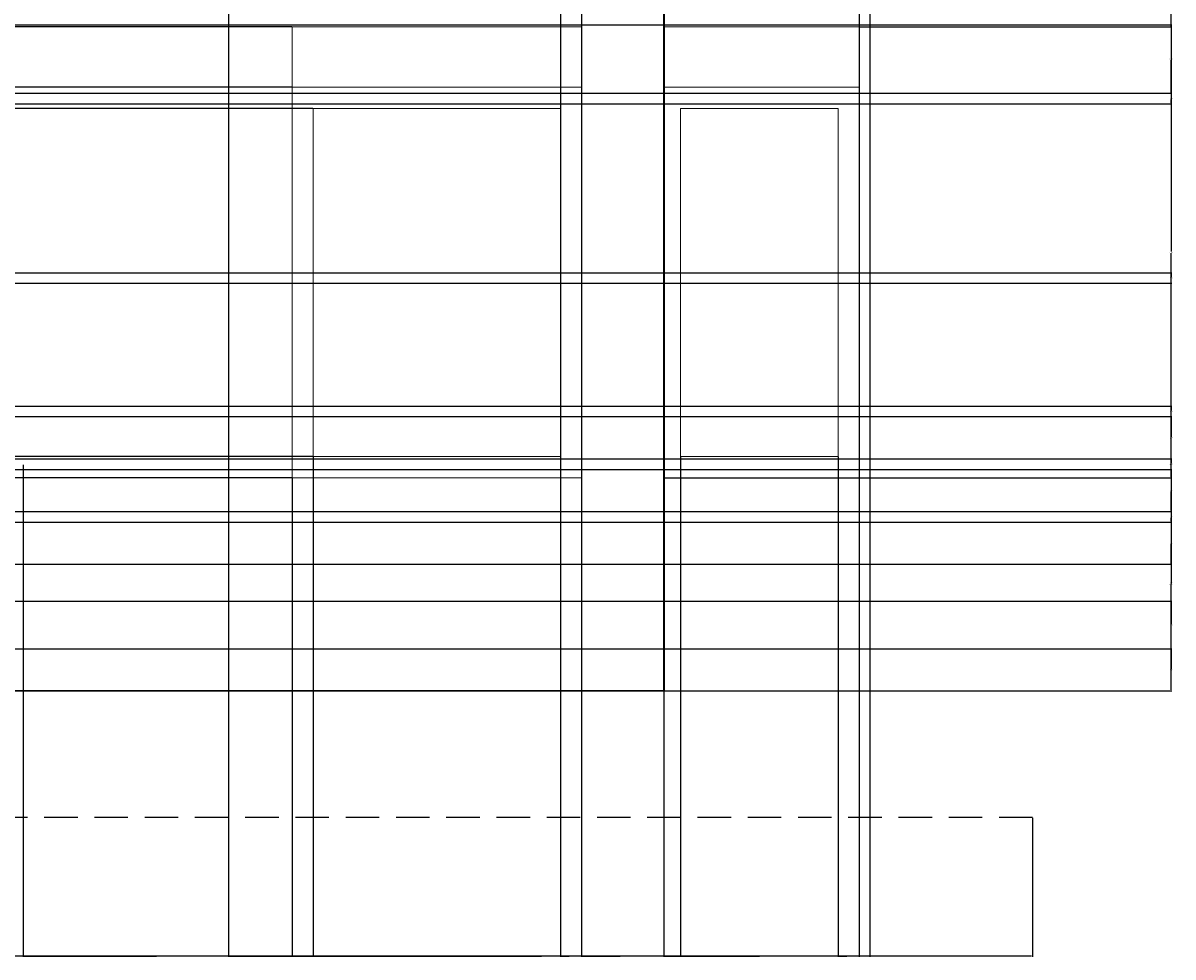
# Model space of a CAD drawing. Units: inches. Extents: x 1817 to 2378, y 1915 to 2370.
# Tile 6 of 8: x 2160 to 2378, y 1915 to 2092. Entities that reach past the tile are written whole.
import ezdxf

# ---------------------------------------------------------------- set-up
doc = ezdxf.new("R2010")
doc.units = ezdxf.units.IN
doc.linetypes.add('DASHED', pattern=[19.05, 12.7, -6.35])
doc.linetypes.add('DASHED2', pattern=[9.525, 6.35, -3.175])
for name, color, linetype, lineweight in [('A-ANNO-DIMS', 2, 'Continuous', 18), ('A-ELEV', 7, 'Continuous', 35), ('A-ELEV-HIDN', 8, 'DASHED', 18), ('A-GLAZ', 4, 'Continuous', 18), ('C-TOPO', 8, 'DASHED2', 25)]:
    doc.layers.add(name, color=color, linetype=linetype, lineweight=lineweight)
doc.styles.get("Standard").update_dxf_attribs({"font": 'arial.ttf'})
doc.dimstyles.get("Standard").update_dxf_attribs({"dimtxt": 0.18, "dimasz": 0.18, "dimexe": 0.18, "dimexo": 0.0625, "dimgap": 0.09, "dimtad": 0, "dimtih": 1, "dimtoh": 1, "dimdec": 4, "dimzin": 0, "dimdsep": 46, "dimtxsty": 'Standard', "dimcen": 0.09, "dimadec": 0, "dimazin": 0, "dimtfac": 1, "dimtdec": 4, "dimtofl": 0, "dimtmove": 0, "dimatfit": 3, "dimfxl": 1, "dimtolj": 1, "dimtzin": 0, "dimarcsym": 0})

# ---------------------------------------------------------------- blocks, each defined once
blk = doc.blocks.new('*D19')
at = {"layer": 'A-ANNO-DIMS', "color": 0, "lineweight": -2, "transparency": 16777216}
for p, q in [((2159.62, 2008.38), (2159.62, 1915.08)), ((2210.62, 2005.87), (2210.62, 1915.08)), ((2159.8, 1915.26), (2184.92, 1915.26)), ((2210.44, 1915.26), (2185.32, 1915.26))]:
    blk.add_line(p, q, dxfattribs=at)
at = {"layer": 'A-ANNO-DIMS', "color": 0, "transparency": 16777216}
for points in [[(2159.8, 1915.29), (2159.8, 1915.23), (2159.62, 1915.26)], [(2210.44, 1915.29), (2210.44, 1915.23), (2210.62, 1915.26)]]:
    blk.add_solid(points, dxfattribs=at)
at = {"layer": 'Defpoints', "color": 0, "transparency": 16777216}
for p in [(2159.62, 2008.45), (2210.62, 2005.93), (2210.62, 1915.26)]:
    blk.add_point(p, dxfattribs=at)
at = {"layer": 'A-ANNO-DIMS', "color": 0, "transparency": 16777216, "insert": (2185.12, 1915.26), "char_height": 0.18, "attachment_point": 5}
blk.add_mtext('\\A1;51', dxfattribs=at)
blk = doc.blocks.new('*D20')
at = {"layer": 'A-ANNO-DIMS', "color": 0, "lineweight": -2, "transparency": 16777216}
for p, q in [((2210.62, 2005.87), (2210.62, 1915.08)), ((2265.49, 2005.87), (2265.49, 1915.08)), ((2210.8, 1915.26), (2237.66, 1915.26)), ((2265.31, 1915.26), (2238.45, 1915.26))]:
    blk.add_line(p, q, dxfattribs=at)
at = {"layer": 'A-ANNO-DIMS', "color": 0, "transparency": 16777216}
for points in [[(2210.8, 1915.29), (2210.8, 1915.23), (2210.62, 1915.26)], [(2265.31, 1915.29), (2265.31, 1915.23), (2265.49, 1915.26)]]:
    blk.add_solid(points, dxfattribs=at)
at = {"layer": 'Defpoints', "color": 0, "transparency": 16777216}
for p in [(2210.62, 2005.93), (2265.49, 2005.93), (2265.49, 1915.26)]:
    blk.add_point(p, dxfattribs=at)
at = {"layer": 'A-ANNO-DIMS', "color": 0, "transparency": 16777216, "insert": (2238.05, 1915.26), "char_height": 0.18, "attachment_point": 5}
blk.add_mtext('\\A1;54.87', dxfattribs=at)
blk = doc.blocks.new('*D21')
at = {"layer": 'A-ANNO-DIMS', "color": 0, "lineweight": -2, "transparency": 16777216}
for p, q in [((2265.49, 2005.87), (2265.49, 1915.08)), ((2281.08, 2005.87), (2281.08, 1915.08)), ((2265.67, 1915.26), (2272.83, 1915.26)), ((2280.9, 1915.26), (2273.74, 1915.26))]:
    blk.add_line(p, q, dxfattribs=at)
at = {"layer": 'A-ANNO-DIMS', "color": 0, "transparency": 16777216}
for points in [[(2265.67, 1915.29), (2265.67, 1915.23), (2265.49, 1915.26)], [(2280.9, 1915.29), (2280.9, 1915.23), (2281.08, 1915.26)]]:
    blk.add_solid(points, dxfattribs=at)
at = {"layer": 'Defpoints', "color": 0, "transparency": 16777216}
for p in [(2265.49, 2005.93), (2281.08, 2005.93), (2281.08, 1915.26)]:
    blk.add_point(p, dxfattribs=at)
at = {"layer": 'A-ANNO-DIMS', "color": 0, "transparency": 16777216, "insert": (2273.29, 1915.26), "char_height": 0.18, "attachment_point": 5}
blk.add_mtext('\\A1;15.596', dxfattribs=at)
blk = doc.blocks.new('*D22')
at = {"layer": 'A-ANNO-DIMS', "color": 0, "lineweight": -2, "transparency": 16777216}
for p, q in [((2281.08, 2005.87), (2281.08, 1915.08)), ((2318.11, 2005.87), (2318.11, 1915.08)), ((2281.26, 1915.26), (2299.2, 1915.26)), ((2317.93, 1915.26), (2299.99, 1915.26))]:
    blk.add_line(p, q, dxfattribs=at)
at = {"layer": 'A-ANNO-DIMS', "color": 0, "transparency": 16777216}
for points in [[(2281.26, 1915.29), (2281.26, 1915.23), (2281.08, 1915.26)], [(2317.93, 1915.29), (2317.93, 1915.23), (2318.11, 1915.26)]]:
    blk.add_solid(points, dxfattribs=at)
at = {"layer": 'Defpoints', "color": 0, "transparency": 16777216}
for p in [(2281.08, 2005.93), (2318.11, 2005.93), (2318.11, 1915.26)]:
    blk.add_point(p, dxfattribs=at)
at = {"layer": 'A-ANNO-DIMS', "color": 0, "transparency": 16777216, "insert": (2299.6, 1915.26), "char_height": 0.18, "attachment_point": 5}
blk.add_mtext('\\A1;37.02', dxfattribs=at)
blk = doc.blocks.new('*D23')
at = {"layer": 'A-ANNO-DIMS', "color": 0, "lineweight": -2, "transparency": 16777216}
for p, q in [((2320.11, 2156.45), (2320.11, 1915.08)), ((1867.08, 1965.45), (1867.08, 1915.08)), ((1867.26, 1915.26), (2093.3, 1915.26)), ((2319.93, 1915.26), (2093.89, 1915.26))]:
    blk.add_line(p, q, dxfattribs=at)
at = {"layer": 'A-ANNO-DIMS', "color": 0, "transparency": 16777216}
for points in [[(1867.26, 1915.29), (1867.26, 1915.23), (1867.08, 1915.26)], [(2319.93, 1915.29), (2319.93, 1915.23), (2320.11, 1915.26)]]:
    blk.add_solid(points, dxfattribs=at)
at = {"layer": 'Defpoints', "color": 0, "transparency": 16777216}
for p in [(2320.11, 2156.51), (1867.08, 1965.51), (2320.11, 1915.26)]:
    blk.add_point(p, dxfattribs=at)
at = {"layer": 'A-ANNO-DIMS', "color": 0, "transparency": 16777216, "insert": (2093.6, 1915.26), "char_height": 0.18, "attachment_point": 5}
blk.add_mtext('\\A1;453', dxfattribs=at)
blk = doc.blocks.new('*D24')
at = {"layer": 'A-ANNO-DIMS', "color": 0, "lineweight": -2, "transparency": 16777216}
for p, q in [((2198.59, 2103.51), (2198.59, 1915.08)), ((2318.11, 2103.51), (2318.11, 1915.08)), ((2198.77, 1915.26), (2257.89, 1915.26)), ((2317.93, 1915.26), (2258.8, 1915.26))]:
    blk.add_line(p, q, dxfattribs=at)
at = {"layer": 'A-ANNO-DIMS', "color": 0, "transparency": 16777216}
for points in [[(2198.77, 1915.29), (2198.77, 1915.23), (2198.59, 1915.26)], [(2317.93, 1915.29), (2317.93, 1915.23), (2318.11, 1915.26)]]:
    blk.add_solid(points, dxfattribs=at)
at = {"layer": 'Defpoints', "color": 0, "transparency": 16777216}
for p in [(2198.59, 2103.57), (2318.11, 2103.57), (2318.11, 1915.26)]:
    blk.add_point(p, dxfattribs=at)
at = {"layer": 'A-ANNO-DIMS', "color": 0, "transparency": 16777216, "insert": (2258.35, 1915.26), "char_height": 0.18, "attachment_point": 5}
blk.add_mtext('\\A1;119.52', dxfattribs=at)
blk = doc.blocks.new('*D69')
at = {"layer": 'A-ANNO-DIMS', "color": 0, "lineweight": -2, "transparency": 16777216}
for p, q in [((2281.15, 2005.93), (2377.4, 2005.93)), ((2377.22, 2005.75), (2377.22, 1985.9)), ((2377.22, 1965.69), (2377.22, 1985.54)), ((2281.15, 1965.51), (2377.4, 1965.51))]:
    blk.add_line(p, q, dxfattribs=at)
at = {"layer": 'A-ANNO-DIMS', "color": 0, "transparency": 16777216}
for points in [[(2377.19, 2005.75), (2377.25, 2005.75), (2377.22, 2005.93)], [(2377.19, 1965.69), (2377.25, 1965.69), (2377.22, 1965.51)]]:
    blk.add_solid(points, dxfattribs=at)
at = {"layer": 'Defpoints', "color": 0, "transparency": 16777216}
for p in [(2281.08, 2005.93), (2377.22, 2005.93), (2281.08, 1965.51)]:
    blk.add_point(p, dxfattribs=at)
at = {"layer": 'A-ANNO-DIMS', "color": 0, "transparency": 16777216, "insert": (2377.22, 1985.72), "char_height": 0.18, "attachment_point": 5}
blk.add_mtext('\\A1;40.42', dxfattribs=at)
blk = doc.blocks.new('*D70')
at = {"layer": 'A-ANNO-DIMS', "color": 0, "lineweight": -2, "transparency": 16777216}
for p, q in [((2318.17, 2091.36), (2377.4, 2091.36)), ((2377.22, 2091.18), (2377.22, 2048.83)), ((2377.22, 2006.11), (2377.22, 2048.47)), ((2281.15, 2005.93), (2377.4, 2005.93))]:
    blk.add_line(p, q, dxfattribs=at)
at = {"layer": 'A-ANNO-DIMS', "color": 0, "transparency": 16777216}
for points in [[(2377.19, 2091.18), (2377.25, 2091.18), (2377.22, 2091.36)], [(2377.19, 2006.11), (2377.25, 2006.11), (2377.22, 2005.93)]]:
    blk.add_solid(points, dxfattribs=at)
at = {"layer": 'Defpoints', "color": 0, "transparency": 16777216}
for p in [(2318.11, 2091.36), (2377.22, 2091.36), (2281.08, 2005.93)]:
    blk.add_point(p, dxfattribs=at)
at = {"layer": 'A-ANNO-DIMS', "color": 0, "transparency": 16777216, "insert": (2377.22, 2048.65), "char_height": 0.18, "attachment_point": 5}
blk.add_mtext('\\A1;85.43', dxfattribs=at)
blk = doc.blocks.new('*D71')
at = {"layer": 'A-ANNO-DIMS', "color": 0, "lineweight": -2, "transparency": 16777216}
for p, q in [((2318.17, 2103.57), (2377.4, 2103.57)), ((2377.22, 2103.39), (2377.22, 2097.65)), ((2377.22, 2091.54), (2377.22, 2097.29)), ((2318.17, 2091.36), (2377.4, 2091.36))]:
    blk.add_line(p, q, dxfattribs=at)
at = {"layer": 'A-ANNO-DIMS', "color": 0, "transparency": 16777216}
for points in [[(2377.19, 2103.39), (2377.25, 2103.39), (2377.22, 2103.57)], [(2377.19, 2091.54), (2377.25, 2091.54), (2377.22, 2091.36)]]:
    blk.add_solid(points, dxfattribs=at)
at = {"layer": 'Defpoints', "color": 0, "transparency": 16777216}
for p in [(2318.11, 2103.57), (2377.22, 2103.57), (2318.11, 2091.36)]:
    blk.add_point(p, dxfattribs=at)
at = {"layer": 'A-ANNO-DIMS', "color": 0, "transparency": 16777216, "insert": (2377.22, 2097.47), "char_height": 0.18, "attachment_point": 5}
blk.add_mtext('\\A1;12.207', dxfattribs=at)
blk = doc.blocks.new('*D80')
at = {"layer": 'A-ANNO-DIMS', "color": 0, "lineweight": -2, "transparency": 16777216}
for p, q in [((2123.56, 2008.45), (1817.4, 2008.45)), ((1817.58, 2008.27), (1817.58, 1987.16)), ((1817.58, 1965.69), (1817.58, 1986.8)), ((2281.02, 1965.51), (1817.4, 1965.51))]:
    blk.add_line(p, q, dxfattribs=at)
at = {"layer": 'A-ANNO-DIMS', "color": 0, "transparency": 16777216}
for points in [[(1817.55, 2008.27), (1817.61, 2008.27), (1817.58, 2008.45)], [(1817.55, 1965.69), (1817.61, 1965.69), (1817.58, 1965.51)]]:
    blk.add_solid(points, dxfattribs=at)
at = {"layer": 'Defpoints', "color": 0, "transparency": 16777216}
for p in [(1817.58, 2008.45), (2123.62, 2008.45), (2281.08, 1965.51)]:
    blk.add_point(p, dxfattribs=at)
at = {"layer": 'A-ANNO-DIMS', "color": 0, "transparency": 16777216, "insert": (1817.58, 1986.98), "char_height": 0.18, "attachment_point": 5}
blk.add_mtext('\\A1;42.94', dxfattribs=at)
blk = doc.blocks.new('*D84')
at = {"layer": 'A-ANNO-DIMS', "color": 0, "lineweight": -2, "transparency": 16777216}
for p, q in [((1960.49, 2091.79), (2377.4, 2091.79)), ((2377.22, 2091.61), (2377.22, 2085.47)), ((2377.22, 2078.97), (2377.22, 2085.1)), ((1960.49, 2078.79), (2377.4, 2078.79))]:
    blk.add_line(p, q, dxfattribs=at)
at = {"layer": 'A-ANNO-DIMS', "color": 0, "transparency": 16777216}
for points in [[(2377.19, 2091.61), (2377.25, 2091.61), (2377.22, 2091.79)], [(2377.19, 2078.97), (2377.25, 2078.97), (2377.22, 2078.79)]]:
    blk.add_solid(points, dxfattribs=at)
at = {"layer": 'Defpoints', "color": 0, "transparency": 16777216}
for p in [(1960.43, 2091.79), (1960.43, 2078.79), (2377.22, 2078.79)]:
    blk.add_point(p, dxfattribs=at)
at = {"layer": 'A-ANNO-DIMS', "color": 0, "transparency": 16777216, "insert": (2377.22, 2085.29), "char_height": 0.18, "attachment_point": 5}
blk.add_mtext('\\A1;13.00', dxfattribs=at)
blk = doc.blocks.new('*D85')
at = {"layer": 'A-ANNO-DIMS', "color": 0, "lineweight": -2, "transparency": 16777216}
for p, q in [((1960.49, 2078.79), (2377.4, 2078.79)), ((2377.22, 2078.61), (2377.22, 2077.97)), ((2377.22, 2076.97), (2377.22, 2077.6)), ((1958.49, 2076.79), (2377.4, 2076.79))]:
    blk.add_line(p, q, dxfattribs=at)
at = {"layer": 'A-ANNO-DIMS', "color": 0, "transparency": 16777216}
for points in [[(2377.19, 2078.61), (2377.25, 2078.61), (2377.22, 2078.79)], [(2377.19, 2076.97), (2377.25, 2076.97), (2377.22, 2076.79)]]:
    blk.add_solid(points, dxfattribs=at)
at = {"layer": 'Defpoints', "color": 0, "transparency": 16777216}
for p in [(1960.43, 2078.79), (1958.43, 2076.79), (2377.22, 2076.79)]:
    blk.add_point(p, dxfattribs=at)
at = {"layer": 'A-ANNO-DIMS', "color": 0, "transparency": 16777216, "insert": (2377.22, 2077.79), "char_height": 0.18, "attachment_point": 5}
blk.add_mtext('\\A1;2.00', dxfattribs=at)
blk = doc.blocks.new('*D86')
at = {"layer": 'A-ANNO-DIMS', "color": 0, "lineweight": -2, "transparency": 16777216}
for p, q in [((1958.49, 2044.79), (2377.4, 2044.79)), ((1960.49, 2042.79), (2377.4, 2042.79)), ((2377.22, 2044.61), (2377.22, 2043.97)), ((2377.22, 2042.97), (2377.22, 2043.6))]:
    blk.add_line(p, q, dxfattribs=at)
at = {"layer": 'A-ANNO-DIMS', "color": 0, "transparency": 16777216}
for points in [[(2377.19, 2044.61), (2377.25, 2044.61), (2377.22, 2044.79)], [(2377.19, 2042.97), (2377.25, 2042.97), (2377.22, 2042.79)]]:
    blk.add_solid(points, dxfattribs=at)
at = {"layer": 'Defpoints', "color": 0, "transparency": 16777216}
for p in [(1958.43, 2044.79), (1960.43, 2042.79), (2377.22, 2042.79)]:
    blk.add_point(p, dxfattribs=at)
at = {"layer": 'A-ANNO-DIMS', "color": 0, "transparency": 16777216, "insert": (2377.22, 2043.79), "char_height": 0.18, "attachment_point": 5}
blk.add_mtext('\\A1;2.00', dxfattribs=at)
blk = doc.blocks.new('*D94')
at = {"layer": 'A-ANNO-DIMS', "color": 0, "lineweight": -2, "transparency": 16777216}
for p, q in [((2210.55, 2091.36), (1817.4, 2091.36)), ((1817.58, 2091.18), (1817.58, 2085.83)), ((1817.58, 2080.11), (1817.58, 2085.47)), ((2210.55, 2079.93), (1817.4, 2079.93))]:
    blk.add_line(p, q, dxfattribs=at)
at = {"layer": 'A-ANNO-DIMS', "color": 0, "transparency": 16777216}
for points in [[(1817.55, 2091.18), (1817.61, 2091.18), (1817.58, 2091.36)], [(1817.55, 2080.11), (1817.61, 2080.11), (1817.58, 2079.93)]]:
    blk.add_solid(points, dxfattribs=at)
at = {"layer": 'Defpoints', "color": 0, "transparency": 16777216}
for p in [(2210.62, 2091.36), (1817.58, 2079.93), (2210.62, 2079.93)]:
    blk.add_point(p, dxfattribs=at)
at = {"layer": 'A-ANNO-DIMS', "color": 0, "transparency": 16777216, "insert": (1817.58, 2085.65), "char_height": 0.18, "attachment_point": 5}
blk.add_mtext('\\A1;11.433', dxfattribs=at)
blk = doc.blocks.new('*D95')
at = {"layer": 'A-ANNO-DIMS', "color": 0, "lineweight": -2, "transparency": 16777216}
for p, q in [((2210.55, 2079.93), (1817.4, 2079.93)), ((1817.58, 2079.75), (1817.58, 2078.11)), ((1817.58, 2076.11), (1817.58, 2077.75)), ((2214.55, 2075.93), (1817.4, 2075.93))]:
    blk.add_line(p, q, dxfattribs=at)
at = {"layer": 'A-ANNO-DIMS', "color": 0, "transparency": 16777216}
for points in [[(1817.55, 2079.75), (1817.61, 2079.75), (1817.58, 2079.93)], [(1817.55, 2076.11), (1817.61, 2076.11), (1817.58, 2075.93)]]:
    blk.add_solid(points, dxfattribs=at)
at = {"layer": 'Defpoints', "color": 0, "transparency": 16777216}
for p in [(2210.62, 2079.93), (1817.58, 2075.93), (2214.62, 2075.93)]:
    blk.add_point(p, dxfattribs=at)
at = {"layer": 'A-ANNO-DIMS', "color": 0, "transparency": 16777216, "insert": (1817.58, 2077.93), "char_height": 0.18, "attachment_point": 5}
blk.add_mtext('\\A1;4.00', dxfattribs=at)
blk = doc.blocks.new('*D96')
at = {"layer": 'A-ANNO-DIMS', "color": 0, "lineweight": -2, "transparency": 16777216}
for p, q in [((2214.55, 2009.93), (1817.4, 2009.93)), ((1817.58, 2009.75), (1817.58, 2008.11)), ((1817.58, 2006.11), (1817.58, 2007.75)), ((2210.55, 2005.93), (1817.4, 2005.93))]:
    blk.add_line(p, q, dxfattribs=at)
at = {"layer": 'A-ANNO-DIMS', "color": 0, "transparency": 16777216}
for points in [[(1817.55, 2009.75), (1817.61, 2009.75), (1817.58, 2009.93)], [(1817.55, 2006.11), (1817.61, 2006.11), (1817.58, 2005.93)]]:
    blk.add_solid(points, dxfattribs=at)
at = {"layer": 'Defpoints', "color": 0, "transparency": 16777216}
for p in [(2214.62, 2009.93), (1817.58, 2005.93), (2210.62, 2005.93)]:
    blk.add_point(p, dxfattribs=at)
at = {"layer": 'A-ANNO-DIMS', "color": 0, "transparency": 16777216, "insert": (1817.58, 2007.93), "char_height": 0.18, "attachment_point": 5}
blk.add_mtext('\\A1;4.00', dxfattribs=at)
blk = doc.blocks.new('*D97')
at = {"layer": 'A-ANNO-DIMS', "color": 0, "lineweight": -2, "transparency": 16777216}
for p, q in [((2214.62, 2009.87), (2214.62, 1915.08)), ((2210.62, 2005.87), (2210.62, 1915.08)), ((2210.8, 1915.26), (2212.29, 1915.26)), ((2214.44, 1915.26), (2212.94, 1915.26))]:
    blk.add_line(p, q, dxfattribs=at)
at = {"layer": 'A-ANNO-DIMS', "color": 0, "transparency": 16777216}
for points in [[(2210.8, 1915.29), (2210.8, 1915.23), (2210.62, 1915.26)], [(2214.44, 1915.29), (2214.44, 1915.23), (2214.62, 1915.26)]]:
    blk.add_solid(points, dxfattribs=at)
at = {"layer": 'Defpoints', "color": 0, "transparency": 16777216}
for p in [(2214.62, 2009.93), (2210.62, 2005.93), (2214.62, 1915.26)]:
    blk.add_point(p, dxfattribs=at)
at = {"layer": 'A-ANNO-DIMS', "color": 0, "transparency": 16777216, "insert": (2212.62, 1915.26), "char_height": 0.18, "attachment_point": 5}
blk.add_mtext('\\A1;4.00', dxfattribs=at)
blk = doc.blocks.new('*D98')
at = {"layer": 'A-ANNO-DIMS', "color": 0, "lineweight": -2, "transparency": 16777216}
for p, q in [((2284.27, 2009.87), (2284.27, 1915.08)), ((2281.08, 2005.87), (2281.08, 1915.08)), ((2281.26, 1915.26), (2282.29, 1915.26)), ((2284.09, 1915.26), (2283.07, 1915.26))]:
    blk.add_line(p, q, dxfattribs=at)
at = {"layer": 'A-ANNO-DIMS', "color": 0, "transparency": 16777216}
for points in [[(2281.26, 1915.29), (2281.26, 1915.23), (2281.08, 1915.26)], [(2284.09, 1915.29), (2284.09, 1915.23), (2284.27, 1915.26)]]:
    blk.add_solid(points, dxfattribs=at)
at = {"layer": 'Defpoints', "color": 0, "transparency": 16777216}
for p in [(2284.27, 2009.93), (2281.08, 2005.93), (2284.27, 1915.26)]:
    blk.add_point(p, dxfattribs=at)
at = {"layer": 'A-ANNO-DIMS', "color": 0, "transparency": 16777216, "insert": (2282.68, 1915.26), "char_height": 0.18, "attachment_point": 5}
blk.add_mtext('\\A1;3.188', dxfattribs=at)
blk = doc.blocks.new('*D99')
at = {"layer": 'A-ANNO-DIMS', "color": 0, "lineweight": -2, "transparency": 16777216}
for p, q in [((2314.11, 2009.87), (2314.11, 1915.08)), ((2318.11, 2005.87), (2318.11, 1915.08)), ((2314.29, 1915.26), (2315.78, 1915.26)), ((2317.93, 1915.26), (2316.43, 1915.26))]:
    blk.add_line(p, q, dxfattribs=at)
at = {"layer": 'A-ANNO-DIMS', "color": 0, "transparency": 16777216}
for points in [[(2314.29, 1915.29), (2314.29, 1915.23), (2314.11, 1915.26)], [(2317.93, 1915.29), (2317.93, 1915.23), (2318.11, 1915.26)]]:
    blk.add_solid(points, dxfattribs=at)
at = {"layer": 'Defpoints', "color": 0, "transparency": 16777216}
for p in [(2314.11, 2009.93), (2318.11, 2005.93), (2314.11, 1915.26)]:
    blk.add_point(p, dxfattribs=at)
at = {"layer": 'A-ANNO-DIMS', "color": 0, "transparency": 16777216, "insert": (2316.11, 1915.26), "char_height": 0.18, "attachment_point": 5}
blk.add_mtext('\\A1;4.00', dxfattribs=at)
blk = doc.blocks.new('*D106')
at = {"layer": 'A-ANNO-DIMS', "color": 0, "lineweight": -2, "transparency": 16777216}
for p, q in [((2261.49, 2156.45), (2261.49, 1915.08)), ((2265.49, 2156.45), (2265.49, 1915.08)), ((2261.67, 1915.26), (2263.16, 1915.26)), ((2265.31, 1915.26), (2263.82, 1915.26))]:
    blk.add_line(p, q, dxfattribs=at)
at = {"layer": 'A-ANNO-DIMS', "color": 0, "transparency": 16777216}
for points in [[(2261.67, 1915.29), (2261.67, 1915.23), (2261.49, 1915.26)], [(2265.31, 1915.29), (2265.31, 1915.23), (2265.49, 1915.26)]]:
    blk.add_solid(points, dxfattribs=at)
at = {"layer": 'Defpoints', "color": 0, "transparency": 16777216}
for p in [(2261.49, 2156.51), (2265.49, 2156.51), (2261.49, 1915.26)]:
    blk.add_point(p, dxfattribs=at)
at = {"layer": 'A-ANNO-DIMS', "color": 0, "transparency": 16777216, "insert": (2263.49, 1915.26), "char_height": 0.18, "attachment_point": 5}
blk.add_mtext('\\A1;4.00', dxfattribs=at)
blk = doc.blocks.new('*D107')
at = {"layer": 'A-ANNO-DIMS', "color": 0, "lineweight": -2, "transparency": 16777216}
for p, q in [((1903.15, 2019.51), (2377.4, 2019.51)), ((2377.22, 2019.33), (2377.22, 2018.69)), ((1903.15, 2017.51), (2377.4, 2017.51)), ((2377.22, 2017.69), (2377.22, 2018.33))]:
    blk.add_line(p, q, dxfattribs=at)
at = {"layer": 'A-ANNO-DIMS', "color": 0, "transparency": 16777216}
for points in [[(2377.19, 2019.33), (2377.25, 2019.33), (2377.22, 2019.51)], [(2377.19, 2017.69), (2377.25, 2017.69), (2377.22, 2017.51)]]:
    blk.add_solid(points, dxfattribs=at)
at = {"layer": 'Defpoints', "color": 0, "transparency": 16777216}
for p in [(1903.08, 2019.51), (1903.08, 2017.51), (2377.22, 2017.51)]:
    blk.add_point(p, dxfattribs=at)
at = {"layer": 'A-ANNO-DIMS', "color": 0, "transparency": 16777216, "insert": (2377.22, 2018.51), "char_height": 0.18, "attachment_point": 5}
blk.add_mtext('\\A1;2.00', dxfattribs=at)
blk = doc.blocks.new('*D108')
at = {"layer": 'A-ANNO-DIMS', "color": 0, "lineweight": -2, "transparency": 16777216}
for p, q in [((1903.15, 2017.51), (2377.4, 2017.51)), ((2377.22, 2017.33), (2377.22, 2013.69)), ((2377.22, 2009.69), (2377.22, 2013.33)), ((1903.15, 2009.51), (2377.4, 2009.51))]:
    blk.add_line(p, q, dxfattribs=at)
at = {"layer": 'A-ANNO-DIMS', "color": 0, "transparency": 16777216}
for points in [[(2377.19, 2017.33), (2377.25, 2017.33), (2377.22, 2017.51)], [(2377.19, 2009.69), (2377.25, 2009.69), (2377.22, 2009.51)]]:
    blk.add_solid(points, dxfattribs=at)
at = {"layer": 'Defpoints', "color": 0, "transparency": 16777216}
for p in [(1903.08, 2017.51), (1903.08, 2009.51), (2377.22, 2009.51)]:
    blk.add_point(p, dxfattribs=at)
at = {"layer": 'A-ANNO-DIMS', "color": 0, "transparency": 16777216, "insert": (2377.22, 2013.51), "char_height": 0.18, "attachment_point": 5}
blk.add_mtext('\\A1;8.00', dxfattribs=at)
blk = doc.blocks.new('*D109')
at = {"layer": 'A-ANNO-DIMS', "color": 0, "lineweight": -2, "transparency": 16777216}
for p, q in [((1903.15, 2009.51), (2377.4, 2009.51)), ((2377.22, 2009.33), (2377.22, 2008.69)), ((2377.22, 2007.69), (2377.22, 2008.33)), ((1903.15, 2007.51), (2377.4, 2007.51))]:
    blk.add_line(p, q, dxfattribs=at)
at = {"layer": 'A-ANNO-DIMS', "color": 0, "transparency": 16777216}
for points in [[(2377.19, 2009.33), (2377.25, 2009.33), (2377.22, 2009.51)], [(2377.19, 2007.69), (2377.25, 2007.69), (2377.22, 2007.51)]]:
    blk.add_solid(points, dxfattribs=at)
at = {"layer": 'Defpoints', "color": 0, "transparency": 16777216}
for p in [(1903.08, 2009.51), (1903.08, 2007.51), (2377.22, 2007.51)]:
    blk.add_point(p, dxfattribs=at)
at = {"layer": 'A-ANNO-DIMS', "color": 0, "transparency": 16777216, "insert": (2377.22, 2008.51), "char_height": 0.18, "attachment_point": 5}
blk.add_mtext('\\A1;2.00', dxfattribs=at)
blk = doc.blocks.new('*D110')
at = {"layer": 'A-ANNO-DIMS', "color": 0, "lineweight": -2, "transparency": 16777216}
for p, q in [((1903.15, 2007.51), (2377.4, 2007.51)), ((2377.22, 2007.33), (2377.22, 2003.69)), ((2377.22, 1999.69), (2377.22, 2003.33)), ((1903.15, 1999.51), (2377.4, 1999.51))]:
    blk.add_line(p, q, dxfattribs=at)
at = {"layer": 'A-ANNO-DIMS', "color": 0, "transparency": 16777216}
for points in [[(2377.19, 2007.33), (2377.25, 2007.33), (2377.22, 2007.51)], [(2377.19, 1999.69), (2377.25, 1999.69), (2377.22, 1999.51)]]:
    blk.add_solid(points, dxfattribs=at)
at = {"layer": 'Defpoints', "color": 0, "transparency": 16777216}
for p in [(1903.08, 2007.51), (1903.08, 1999.51), (2377.22, 1999.51)]:
    blk.add_point(p, dxfattribs=at)
at = {"layer": 'A-ANNO-DIMS', "color": 0, "transparency": 16777216, "insert": (2377.22, 2003.51), "char_height": 0.18, "attachment_point": 5}
blk.add_mtext('\\A1;8.00', dxfattribs=at)
blk = doc.blocks.new('*D111')
at = {"layer": 'A-ANNO-DIMS', "color": 0, "lineweight": -2, "transparency": 16777216}
for p, q in [((1903.15, 1999.51), (2377.4, 1999.51)), ((2377.22, 1999.33), (2377.22, 1998.69)), ((1903.15, 1997.51), (2377.4, 1997.51)), ((2377.22, 1997.69), (2377.22, 1998.33))]:
    blk.add_line(p, q, dxfattribs=at)
at = {"layer": 'A-ANNO-DIMS', "color": 0, "transparency": 16777216}
for points in [[(2377.19, 1999.33), (2377.25, 1999.33), (2377.22, 1999.51)], [(2377.19, 1997.69), (2377.25, 1997.69), (2377.22, 1997.51)]]:
    blk.add_solid(points, dxfattribs=at)
at = {"layer": 'Defpoints', "color": 0, "transparency": 16777216}
for p in [(1903.08, 1999.51), (1903.08, 1997.51), (2377.22, 1997.51)]:
    blk.add_point(p, dxfattribs=at)
at = {"layer": 'A-ANNO-DIMS', "color": 0, "transparency": 16777216, "insert": (2377.22, 1998.51), "char_height": 0.18, "attachment_point": 5}
blk.add_mtext('\\A1;2.00', dxfattribs=at)
blk = doc.blocks.new('*D112')
at = {"layer": 'A-ANNO-DIMS', "color": 0, "lineweight": -2, "transparency": 16777216}
for p, q in [((1903.15, 1997.51), (2377.4, 1997.51)), ((2377.22, 1997.33), (2377.22, 1993.69)), ((2377.22, 1989.69), (2377.22, 1993.33)), ((1903.15, 1989.51), (2377.4, 1989.51))]:
    blk.add_line(p, q, dxfattribs=at)
at = {"layer": 'A-ANNO-DIMS', "color": 0, "transparency": 16777216}
for points in [[(2377.19, 1997.33), (2377.25, 1997.33), (2377.22, 1997.51)], [(2377.19, 1989.69), (2377.25, 1989.69), (2377.22, 1989.51)]]:
    blk.add_solid(points, dxfattribs=at)
at = {"layer": 'Defpoints', "color": 0, "transparency": 16777216}
for p in [(1903.08, 1997.51), (1903.08, 1989.51), (2377.22, 1989.51)]:
    blk.add_point(p, dxfattribs=at)
at = {"layer": 'A-ANNO-DIMS', "color": 0, "transparency": 16777216, "insert": (2377.22, 1993.51), "char_height": 0.18, "attachment_point": 5}
blk.add_mtext('\\A1;8.00', dxfattribs=at)
blk = doc.blocks.new('*D113')
at = {"layer": 'A-ANNO-DIMS', "color": 0, "lineweight": -2, "transparency": 16777216}
for p, q in [((1903.15, 1989.51), (2377.4, 1989.51)), ((2377.22, 1989.33), (2377.22, 1986.19)), ((2377.22, 1982.69), (2377.22, 1985.83)), ((1903.15, 1982.51), (2377.4, 1982.51))]:
    blk.add_line(p, q, dxfattribs=at)
at = {"layer": 'A-ANNO-DIMS', "color": 0, "transparency": 16777216}
for points in [[(2377.19, 1989.33), (2377.25, 1989.33), (2377.22, 1989.51)], [(2377.19, 1982.69), (2377.25, 1982.69), (2377.22, 1982.51)]]:
    blk.add_solid(points, dxfattribs=at)
at = {"layer": 'Defpoints', "color": 0, "transparency": 16777216}
for p in [(1903.08, 1989.51), (1903.08, 1982.51), (2377.22, 1982.51)]:
    blk.add_point(p, dxfattribs=at)
at = {"layer": 'A-ANNO-DIMS', "color": 0, "transparency": 16777216, "insert": (2377.22, 1986.01), "char_height": 0.18, "attachment_point": 5}
blk.add_mtext('\\A1;7.00', dxfattribs=at)
blk = doc.blocks.new('*D114')
at = {"layer": 'A-ANNO-DIMS', "color": 0, "lineweight": -2, "transparency": 16777216}
for p, q in [((1903.15, 1982.51), (2377.4, 1982.51)), ((2377.22, 1982.33), (2377.22, 1978.19)), ((2377.22, 1973.69), (2377.22, 1977.83)), ((1903.15, 1973.51), (2377.4, 1973.51))]:
    blk.add_line(p, q, dxfattribs=at)
at = {"layer": 'A-ANNO-DIMS', "color": 0, "transparency": 16777216}
for points in [[(2377.19, 1982.33), (2377.25, 1982.33), (2377.22, 1982.51)], [(2377.19, 1973.69), (2377.25, 1973.69), (2377.22, 1973.51)]]:
    blk.add_solid(points, dxfattribs=at)
at = {"layer": 'Defpoints', "color": 0, "transparency": 16777216}
for p in [(1903.08, 1982.51), (1903.08, 1973.51), (2377.22, 1973.51)]:
    blk.add_point(p, dxfattribs=at)
at = {"layer": 'A-ANNO-DIMS', "color": 0, "transparency": 16777216, "insert": (2377.22, 1978.01), "char_height": 0.18, "attachment_point": 5}
blk.add_mtext('\\A1;9.00', dxfattribs=at)
blk = doc.blocks.new('*D115')
at = {"layer": 'A-ANNO-DIMS', "color": 0, "lineweight": -2, "transparency": 16777216}
for p, q in [((1903.15, 1973.51), (2377.4, 1973.51)), ((2377.22, 1973.33), (2377.22, 1969.69)), ((2377.22, 1965.69), (2377.22, 1969.33)), ((1903.15, 1965.51), (2377.4, 1965.51))]:
    blk.add_line(p, q, dxfattribs=at)
at = {"layer": 'A-ANNO-DIMS', "color": 0, "transparency": 16777216}
for points in [[(2377.19, 1973.33), (2377.25, 1973.33), (2377.22, 1973.51)], [(2377.19, 1965.69), (2377.25, 1965.69), (2377.22, 1965.51)]]:
    blk.add_solid(points, dxfattribs=at)
at = {"layer": 'Defpoints', "color": 0, "transparency": 16777216}
for p in [(1903.08, 1973.51), (1903.08, 1965.51), (2377.22, 1965.51)]:
    blk.add_point(p, dxfattribs=at)
at = {"layer": 'A-ANNO-DIMS', "color": 0, "transparency": 16777216, "insert": (2377.22, 1969.51), "char_height": 0.18, "attachment_point": 5}
blk.add_mtext('\\A1;8.00', dxfattribs=at)
blk = doc.blocks.new('*D118')
at = {"layer": 'A-ANNO-DIMS', "color": 0, "lineweight": -2, "transparency": 16777216}
for p, q in [((1843.83, 1941.45), (1843.83, 1915.08)), ((2350.97, 1941.45), (2350.97, 1915.08)), ((1844.01, 1915.26), (2096.94, 1915.26)), ((2350.79, 1915.26), (2097.86, 1915.26))]:
    blk.add_line(p, q, dxfattribs=at)
at = {"layer": 'A-ANNO-DIMS', "color": 0, "transparency": 16777216}
for points in [[(1844.01, 1915.29), (1844.01, 1915.23), (1843.83, 1915.26)], [(2350.79, 1915.29), (2350.79, 1915.23), (2350.97, 1915.26)]]:
    blk.add_solid(points, dxfattribs=at)
at = {"layer": 'Defpoints', "color": 0, "transparency": 16777216}
for p in [(1843.83, 1941.51), (2350.97, 1941.51), (2350.97, 1915.26)]:
    blk.add_point(p, dxfattribs=at)
at = {"layer": 'A-ANNO-DIMS', "color": 0, "transparency": 16777216, "insert": (2097.4, 1915.26), "char_height": 0.18, "attachment_point": 5}
blk.add_mtext('\\A1;507.13', dxfattribs=at)
blk = doc.blocks.new('*D119')
at = {"layer": 'A-ANNO-DIMS', "color": 0, "lineweight": -2, "transparency": 16777216}
for p, q in [((1903.08, 1989.57), (1903.08, 2369.94)), ((1903.26, 2369.76), (2091.62, 2369.76)), ((2280.9, 2369.76), (2092.55, 2369.76)), ((2281.08, 1989.57), (2281.08, 2369.94))]:
    blk.add_line(p, q, dxfattribs=at)
at = {"layer": 'A-ANNO-DIMS', "color": 0, "transparency": 16777216}
for points in [[(1903.26, 2369.79), (1903.26, 2369.73), (1903.08, 2369.76)], [(2280.9, 2369.79), (2280.9, 2369.73), (2281.08, 2369.76)]]:
    blk.add_solid(points, dxfattribs=at)
at = {"layer": 'Defpoints', "color": 0, "transparency": 16777216}
for p in [(2281.08, 2369.76), (1903.08, 1989.51), (2281.08, 1989.51)]:
    blk.add_point(p, dxfattribs=at)
at = {"layer": 'A-ANNO-DIMS', "color": 0, "transparency": 16777216, "insert": (2092.08, 2369.76), "char_height": 0.18, "attachment_point": 5}
blk.add_mtext('\\A1;378.00', dxfattribs=at)

msp = doc.modelspace()

# ---------------------------------------------------------------- linework, layer by layer
at = {"layer": 'A-ELEV'}
msp.add_line((2281.0849, 2251.5087), (2281.0849, 1965.5087), dxfattribs=at)
at = {"layer": 'A-ELEV-HIDN'}
msp.add_line((2281.0849, 1989.5087), (1903.0849, 1989.5087), dxfattribs=at)
at = {"layer": 'A-GLAZ'}
for p, q in [((2210.6163, 2079.9313), (2210.6163, 2091.3647)), ((2210.6163, 2091.3647), (2265.4884, 2091.3647)), ((2265.4884, 2079.9313), (2265.4884, 2091.3647)), ((2281.0849, 2091.3647), (2318.1054, 2091.3647)), ((2318.1054, 2091.3647), (2318.1054, 2005.9313)), ((2210.6163, 2079.9313), (2265.4884, 2079.9313)), ((2210.6163, 2005.9313), (2210.6163, 2079.9313)), ((2210.6163, 2079.9313), (2265.4884, 2079.9313)), ((2265.4884, 2079.9313), (2265.4884, 2005.9313)), ((2281.0849, 2079.9313), (2318.1054, 2079.9313)), ((2282.2729, 2079.9313), (2318.1054, 2079.9313)), ((2214.6163, 2075.9313), (2261.4884, 2075.9313)), ((2214.6163, 2009.9313), (2214.6163, 2075.9313)), ((2261.4884, 2075.9313), (2261.4884, 2009.9313)), ((2284.2729, 2075.9313), (2314.1054, 2075.9313)), ((2284.2729, 2009.9313), (2284.2729, 2075.9313)), ((2314.1054, 2075.9313), (2314.1054, 2009.9313)), ((2214.6163, 2009.9313), (2261.4884, 2009.9313)), ((2284.2729, 2009.9313), (2314.1054, 2009.9313)), ((2210.6163, 2005.9313), (2265.4884, 2005.9313)), ((2281.0849, 2005.9313), (2318.1054, 2005.9313))]:
    msp.add_line(p, q, dxfattribs=at)
at = {"layer": 'C-TOPO'}
for p, q in [((2281.0849, 1965.5087), (1867.0849, 1965.5087)), ((2281.0849, 1965.5087), (2350.9681, 1965.5087)), ((2350.9681, 1941.5087), (1843.834, 1941.5087))]:
    msp.add_line(p, q, dxfattribs=at)

# ---------------------------------------------------------------- dimensions: what is measured, and where the dimension line sits
at = {"layer": 'A-ANNO-DIMS'}
for base, p1, p2, override, picture, middle in [((2281.0849, 2369.7587), (1903.0849, 1989.5087), (2281.0849, 1989.5087), {"dimdec": 2, "dimlfac": 1, "dimrnd": 0, "dimzin": 0, "dimdsep": 46, "dimlunit": 2}, '*D119', (2092.0849, 2369.7587)), ((2320.1054, 1915.2587), (1867.0849, 1965.5087), (2320.1054, 2156.5133), {"dimdec": 0, "dimlfac": 1, "dimrnd": 0, "dimzin": 0, "dimdsep": 46, "dimlunit": 2}, '*D23', (2093.5951, 1915.2587)), ((2261.4884, 1915.2587), (2265.4884, 2156.5133), (2261.4884, 2156.5133), {"dimdec": 2, "dimlfac": 1, "dimrnd": 0, "dimzin": 0, "dimdsep": 46, "dimlunit": 2}, '*D106', (2263.4884, 1915.2587)), ((2318.1054, 1915.2587), (2198.5896, 2103.5721), (2318.1054, 2103.5721), {"dimdec": 2, "dimlfac": 1, "dimrnd": 0, "dimzin": 0, "dimdsep": 46, "dimlunit": 2}, '*D24', (2258.3475, 1915.2587)), ((2214.6163, 1915.2587), (2210.6163, 2005.9313), (2214.6163, 2009.9313), {"dimdec": 2, "dimlfac": 1, "dimrnd": 0, "dimzin": 0, "dimdsep": 46, "dimlunit": 2}, '*D97', (2212.6163, 1915.2587)), ((2284.2729, 1915.2587), (2281.0849, 2005.9313), (2284.2729, 2009.9313), {"dimdec": 3, "dimlfac": 1, "dimrnd": 0, "dimzin": 0, "dimdsep": 46, "dimlunit": 2}, '*D98', (2282.6789, 1915.2587)), ((2314.1054, 1915.2587), (2318.1054, 2005.9313), (2314.1054, 2009.9313), {"dimdec": 2, "dimlfac": 1, "dimrnd": 0, "dimzin": 0, "dimdsep": 46, "dimlunit": 2}, '*D99', (2316.1054, 1915.2587)), ((2210.6163, 1915.2587), (2159.6179, 2008.4468), (2210.6163, 2005.9313), {"dimdec": 0, "dimlfac": 1, "dimrnd": 0, "dimzin": 0, "dimdsep": 46, "dimlunit": 2}, '*D19', (2185.1171, 1915.2587)), ((2265.4884, 1915.2587), (2210.6163, 2005.9313), (2265.4884, 2005.9313), {"dimdec": 2, "dimlfac": 1, "dimrnd": 0, "dimzin": 0, "dimdsep": 46, "dimlunit": 2}, '*D20', (2238.0523, 1915.2587)), ((2281.08485, 1915.25873), (2265.48837, 2005.93129), (2281.08485, 2005.93129), {"dimdec": 3, "dimlfac": 1, "dimrnd": 0, "dimzin": 0, "dimdsep": 46, "dimlunit": 2}, '*D21', (2273.28661, 1915.25873)), ((2318.1054, 1915.2587), (2281.0849, 2005.9313), (2318.1054, 2005.9313), {"dimdec": 2, "dimlfac": 1, "dimrnd": 0, "dimzin": 0, "dimdsep": 46, "dimlunit": 2}, '*D22', (2299.5951, 1915.2587)), ((2350.9681, 1915.2587), (1843.834, 1941.5087), (2350.9681, 1941.5087), {"dimdec": 2, "dimlfac": 1, "dimrnd": 0, "dimzin": 0, "dimdsep": 46, "dimlunit": 2}, '*D118', (2097.401, 1915.2587))]:
    dim = msp.add_linear_dim(base=base, p1=p1, p2=p2, dimstyle='Standard', override=override, dxfattribs=at)
    dim.commit()
    dim.dimension.update_dxf_attribs({"geometry": picture, "text_midpoint": middle})
for base, p1, p2, override, picture, middle in [((2377.2181, 2103.5721), (2318.1054, 2091.3647), (2318.1054, 2103.5721), {"dimdec": 3, "dimlfac": 1, "dimrnd": 0, "dimzin": 0, "dimdsep": 46, "dimlunit": 2}, '*D71', (2377.2181, 2097.4684)), ((1817.584, 2079.9313), (2210.6163, 2091.3647), (2210.6163, 2079.9313), {"dimdec": 3, "dimlfac": 1, "dimrnd": 0, "dimzin": 0, "dimdsep": 46, "dimlunit": 2}, '*D94', (1817.584, 2085.648)), ((2377.2181, 2078.7858), (1960.4258, 2091.7858), (1960.4258, 2078.7858), {"dimdec": 2, "dimlfac": 1, "dimrnd": 0, "dimzin": 0, "dimdsep": 46, "dimlunit": 2}, '*D84', (2377.2181, 2085.2858)), ((2377.2181, 2091.3647), (2281.0849, 2005.9313), (2318.1054, 2091.3647), {"dimdec": 2, "dimlfac": 1, "dimrnd": 0, "dimzin": 0, "dimdsep": 46, "dimlunit": 2}, '*D70', (2377.2181, 2048.648)), ((1817.584, 2075.9313), (2210.6163, 2079.9313), (2214.6163, 2075.9313), {"dimdec": 2, "dimlfac": 1, "dimrnd": 0, "dimzin": 0, "dimdsep": 46, "dimlunit": 2}, '*D95', (1817.584, 2077.9313)), ((2377.2181, 2076.7858), (1960.4258, 2078.7858), (1958.4258, 2076.7858), {"dimdec": 2, "dimlfac": 1, "dimrnd": 0, "dimzin": 0, "dimdsep": 46, "dimlunit": 2}, '*D85', (2377.2181, 2077.7858)), ((2377.2181, 2042.7858), (1958.4258, 2044.7858), (1960.4258, 2042.7858), {"dimdec": 2, "dimlfac": 1, "dimrnd": 0, "dimzin": 0, "dimdsep": 46, "dimlunit": 2}, '*D86', (2377.2181, 2043.7858)), ((2377.2181, 2017.5087), (1903.0849, 2019.5087), (1903.0849, 2017.5087), {"dimdec": 2, "dimlfac": 1, "dimrnd": 0, "dimzin": 0, "dimdsep": 46, "dimlunit": 2}, '*D107', (2377.2181, 2018.5087)), ((2377.2181, 2009.5087), (1903.0849, 2017.5087), (1903.0849, 2009.5087), {"dimdec": 2, "dimlfac": 1, "dimrnd": 0, "dimzin": 0, "dimdsep": 46, "dimlunit": 2}, '*D108', (2377.2181, 2013.5087)), ((1817.584, 2005.9313), (2214.6163, 2009.9313), (2210.6163, 2005.9313), {"dimdec": 2, "dimlfac": 1, "dimrnd": 0, "dimzin": 0, "dimdsep": 46, "dimlunit": 2}, '*D96', (1817.584, 2007.9313)), ((1817.584, 2008.4468), (2281.0849, 1965.5087), (2123.6179, 2008.4468), {"dimdec": 2, "dimlfac": 1, "dimrnd": 0, "dimzin": 0, "dimdsep": 46, "dimlunit": 2}, '*D80', (1817.584, 1986.9777)), ((2377.2181, 2007.5087), (1903.0849, 2009.5087), (1903.0849, 2007.5087), {"dimdec": 2, "dimlfac": 1, "dimrnd": 0, "dimzin": 0, "dimdsep": 46, "dimlunit": 2}, '*D109', (2377.2181, 2008.5087)), ((2377.2181, 1999.5087), (1903.0849, 2007.5087), (1903.0849, 1999.5087), {"dimdec": 2, "dimlfac": 1, "dimrnd": 0, "dimzin": 0, "dimdsep": 46, "dimlunit": 2}, '*D110', (2377.2181, 2003.5087)), ((2377.2181, 2005.9313), (2281.0849, 1965.5087), (2281.0849, 2005.9313), {"dimdec": 2, "dimlfac": 1, "dimrnd": 0, "dimzin": 0, "dimdsep": 46, "dimlunit": 2}, '*D69', (2377.2181, 1985.72)), ((2377.2181, 1997.5087), (1903.0849, 1999.5087), (1903.0849, 1997.5087), {"dimdec": 2, "dimlfac": 1, "dimrnd": 0, "dimzin": 0, "dimdsep": 46, "dimlunit": 2}, '*D111', (2377.2181, 1998.5087)), ((2377.2181, 1989.5087), (1903.0849, 1997.5087), (1903.0849, 1989.5087), {"dimdec": 2, "dimlfac": 1, "dimrnd": 0, "dimzin": 0, "dimdsep": 46, "dimlunit": 2}, '*D112', (2377.2181, 1993.5087)), ((2377.2181, 1982.5087), (1903.0849, 1989.5087), (1903.0849, 1982.5087), {"dimdec": 2, "dimlfac": 1, "dimrnd": 0, "dimzin": 0, "dimdsep": 46, "dimlunit": 2}, '*D113', (2377.2181, 1986.0087)), ((2377.2181, 1973.5087), (1903.0849, 1982.5087), (1903.0849, 1973.5087), {"dimdec": 2, "dimlfac": 1, "dimrnd": 0, "dimzin": 0, "dimdsep": 46, "dimlunit": 2}, '*D114', (2377.2181, 1978.0087)), ((2377.2181, 1965.5087), (1903.0849, 1973.5087), (1903.0849, 1965.5087), {"dimdec": 2, "dimlfac": 1, "dimrnd": 0, "dimzin": 0, "dimdsep": 46, "dimlunit": 2}, '*D115', (2377.2181, 1969.5087))]:
    dim = msp.add_linear_dim(base=base, p1=p1, p2=p2, angle=90, dimstyle='Standard', override=override, dxfattribs=at)
    dim.commit()
    dim.dimension.update_dxf_attribs({"geometry": picture, "text_midpoint": middle})

doc.saveas('drawing.dxf')
